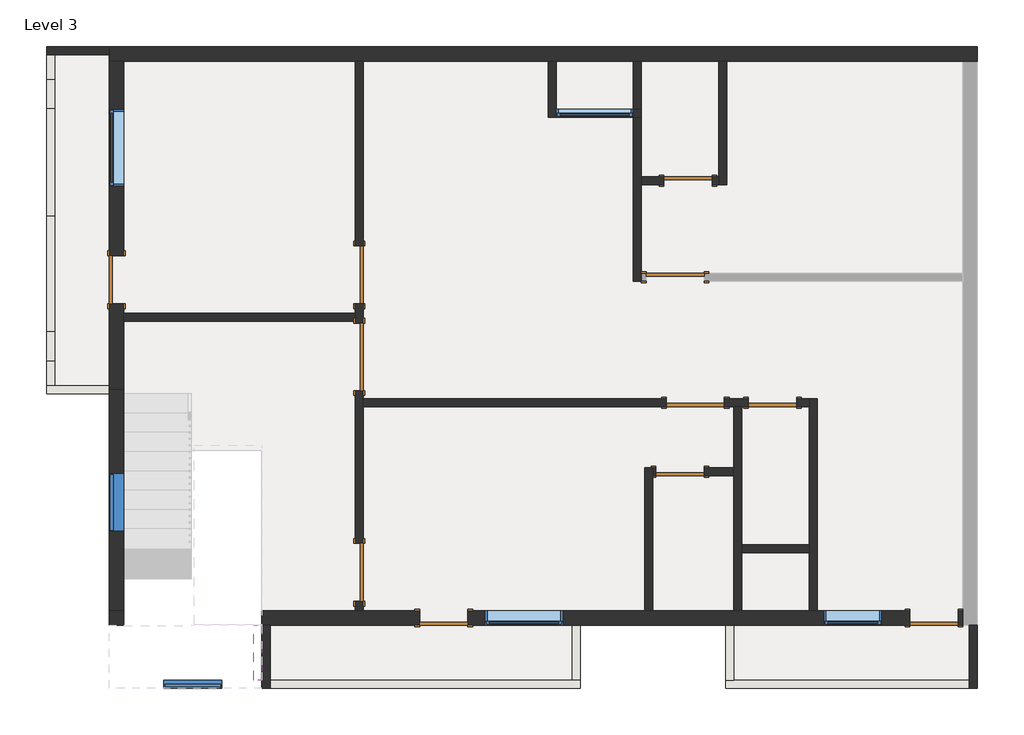
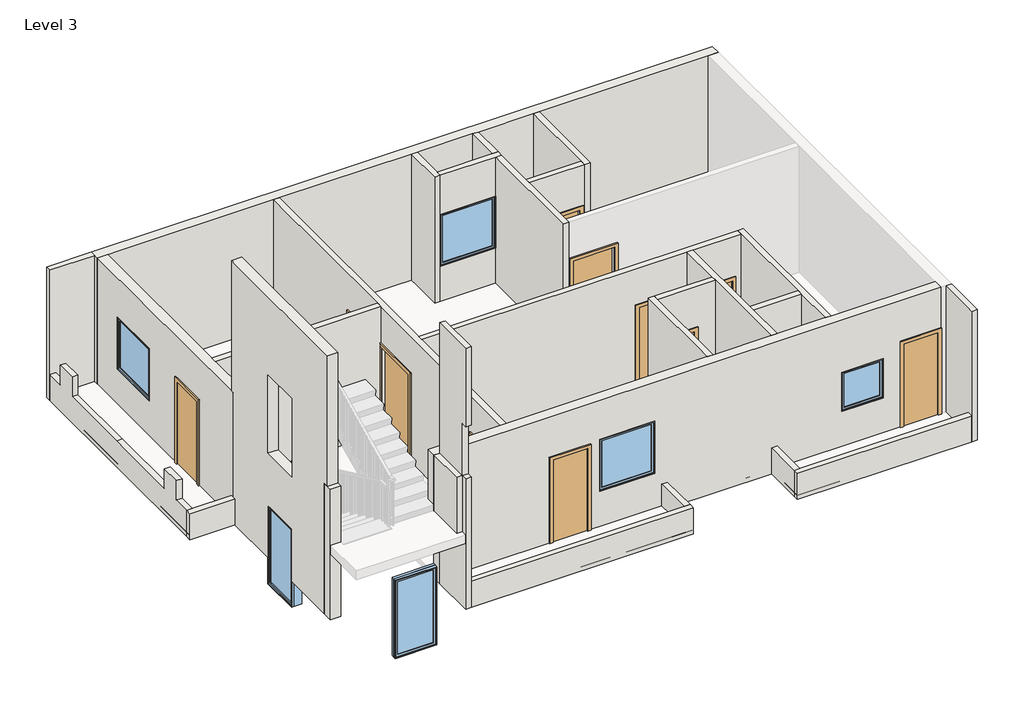
# One storey, part 1 of 2: 29 walls, 11 doors, 6 windows.
"""IFC4 building model written with IfcOpenShell, lengths in millimetres."""

from ifc_helpers import new_model, si_unit, frame, origin, place, context, project, spatial, polyline, outline, extrude, faceted_brep, transform, mapped, element, save
from components import door_1fe7f57d, door_85036156, door_a3eb833a, door_a1797ceb, door_4f94b823, window_6c5853a0, window_7da3115e, window_c796fc87, window_f887c457, window_76f305d9

model = new_model("IFC4")

# Units and contexts
model_context = context("Model", 3, world=origin())
ifc_project = project(units=[si_unit("LENGTHUNIT", "METRE", prefix="MILLI")], contexts=[model_context])

# Site, building, storey
site = spatial("IfcSite", under=ifc_project)
building = spatial("IfcBuilding", under=site)
storey = spatial("IfcBuildingStorey", under=building, Name="Level 3", Elevation=6096.0)

# Doors
placement = place(None, origin())
door_shape = door_1fe7f57d(model_context)
element("IfcDoor", 1, ObjectType="Single-Flush : 30\" x 80\"", at=placement, inside=storey, context=model_context, shape_type="MappedRepresentation", body=[
    mapped(door_shape, transform((-1197.7394758, 10653.5495492, 6096.0), x_axis=(1.0, 0.0, 0.0), y_axis=(0.0, 1.0, 0.0), z_axis=(0.0, 0.0, 1.0))),
])
element("IfcDoor", 2, ObjectType="Single-Flush : 30\" x 80\"", at=placement, inside=storey, context=model_context, shape_type="MappedRepresentation", body=[
    mapped(door_shape, transform((135.7605242, 7148.3495492, 6096.0), x_axis=(-1.0, 0.0, 0.0), y_axis=(0.0, -1.0, 0.0), z_axis=(0.0, 0.0, 1.0))),
])
element("IfcDoor", 3, ObjectType="Single-Flush : 30\" x 80\"", at=placement, inside=storey, context=model_context, shape_type="MappedRepresentation", body=[
    mapped(door_shape, transform((-1324.7394758, 6056.1495492, 6096.0), x_axis=(-1.0, 0.0, 0.0), y_axis=(0.0, -1.0, 0.0), z_axis=(0.0, 0.0, 1.0))),
])
door_2_shape = door_85036156(model_context)
element("IfcDoor", 4, ObjectType="Single-Flush : 30\" x 80\"", at=placement, inside=storey, context=model_context, shape_type="MappedRepresentation", body=[
    mapped(door_2_shape, transform((2688.4605242, 3744.7495492, 6096.0), x_axis=(1.0, 0.0, 0.0), y_axis=(0.0, 1.0, 0.0), z_axis=(0.0, 0.0, 1.0))),
])
element("IfcDoor", 5, ObjectType="Single-Flush : 30\" x 80\"", at=placement, inside=storey, context=model_context, shape_type="MappedRepresentation", body=[
    mapped(door_2_shape, transform((-5058.5394758, 3744.7495492, 6096.0), x_axis=(1.0, 0.0, 0.0), y_axis=(0.0, 1.0, 0.0), z_axis=(0.0, 0.0, 1.0))),
])
element("IfcDoor", 6, ObjectType="Single-Flush : 30\" x 80\"", at=placement, inside=storey, context=model_context, shape_type="MappedRepresentation", body=[
    mapped(door_2_shape, transform((-10227.4394758, 9091.4495492, 6096.0), x_axis=(0.0, -1.0, 0.0), y_axis=(1.0, 0.0, 0.0), z_axis=(0.0, 0.0, 1.0))),
])
door_3_shape = door_a3eb833a(model_context)
element("IfcDoor", 7, ObjectType="Single-Flush : 36\" x 84\"", at=placement, inside=storey, context=model_context, shape_type="MappedRepresentation", body=[
    mapped(door_3_shape, transform((-6392.0394758, 9167.6495492, 6096.0), x_axis=(0.0, 1.0, 0.0), y_axis=(-1.0, 0.0, 0.0), z_axis=(0.0, 0.0, 1.0))),
])
element("IfcDoor", 8, ObjectType="Single-Flush : 36\" x 84\"", at=placement, inside=storey, context=model_context, shape_type="MappedRepresentation", body=[
    mapped(door_3_shape, transform((-1400.9394758, 9129.5495492, 6096.0), x_axis=(-1.0, 0.0, 0.0), y_axis=(0.0, -1.0, 0.0), z_axis=(0.0, 0.0, 1.0))),
])
element("IfcDoor", 9, ObjectType="Single-Flush : 36\" x 84\"", at=placement, inside=storey, context=model_context, shape_type="MappedRepresentation", body=[
    mapped(door_3_shape, transform((-1083.4394758, 7148.3495492, 6096.0), x_axis=(1.0, 0.0, 0.0), y_axis=(0.0, 1.0, 0.0), z_axis=(0.0, 0.0, 1.0))),
])
door_4_shape = door_a1797ceb(model_context)
element("IfcDoor", 10, ObjectType="Single-Flush : 36\" x 84\"", at=placement, inside=storey, context=model_context, shape_type="MappedRepresentation", body=[
    mapped(door_4_shape, transform((-6392.0394758, 4468.6495492, 6096.0), x_axis=(0.0, -1.0, 0.0), y_axis=(1.0, 0.0, 0.0), z_axis=(0.0, 0.0, 1.0))),
])
door_5_shape = door_4f94b823(model_context)
element("IfcDoor", 11, ObjectType="Single-Flush : 42\" x 84\" 3,6\"", at=placement, inside=storey, context=model_context, shape_type="MappedRepresentation", body=[
    mapped(door_5_shape, transform((-6392.0394758, 7872.2495492, 6096.0), x_axis=(0.0, -1.0, 0.0), y_axis=(1.0, 0.0, 0.0), z_axis=(0.0, 0.0, 1.0))),
])

# Walls
element("IfcWall", 12, ObjectType="Generic - 5\"", at=placement, inside=storey, context=model_context, shape_type="Brep", body=[
    faceted_brep([(-6328.5394758, 4925.8495492, 6096.0), (-6328.5394758, 7084.8495492, 6096.0), (-6328.5394758, 7211.8495492, 6096.0), (-6328.5394758, 7338.8495492, 6096.0), (-6328.5394758, 7338.8495492, 8229.6), (-6328.5394758, 8405.6495492, 8229.6), (-6328.5394758, 8405.6495492, 6096.0), (-6328.5394758, 8710.4495492, 6096.0), (-6328.5394758, 8710.4495492, 8229.6), (-6328.5394758, 9624.8495492, 8229.6), (-6328.5394758, 9624.8495492, 6096.0), (-6328.5394758, 12545.8495492, 6096.0), (-6328.5394758, 12545.8495492, 9144.0), (-6328.5394758, 7211.8495492, 9144.0), (-6328.5394758, 7084.8495492, 9144.0), (-6328.5394758, 3859.0495492, 9144.0), (-6328.5394758, 3859.0495492, 6096.0), (-6328.5394758, 4011.4495492, 6096.0), (-6328.5394758, 4011.4495492, 8229.6), (-6328.5394758, 4925.8495492, 8229.6), (-6455.5394758, 7338.8495492, 8229.6), (-6455.5394758, 7338.8495492, 6096.0), (-6455.5394758, 4925.8495492, 6096.0), (-6455.5394758, 4925.8495492, 8229.6), (-6455.5394758, 4011.4495492, 8229.6), (-6455.5394758, 4011.4495492, 6096.0), (-6455.5394758, 3859.0495492, 6096.0), (-6455.5394758, 3859.0495492, 9144.0), (-6455.5394758, 8431.0495492, 9144.0), (-6455.5394758, 8558.0495492, 9144.0), (-6455.5394758, 12545.8495492, 9144.0), (-6455.5394758, 12545.8495492, 6096.0), (-6455.5394758, 9624.8495492, 6096.0), (-6455.5394758, 9624.8495492, 8229.6), (-6455.5394758, 8710.4495492, 8229.6), (-6455.5394758, 8710.4495492, 6096.0), (-6455.5394758, 8558.0495492, 6096.0), (-6455.5394758, 8431.0495492, 6096.0), (-6455.5394758, 8405.6495492, 6096.0), (-6455.5394758, 8405.6495492, 8229.6)], [[[0, 1, 2, 3, 4, 5, 6, 7, 8, 9, 10, 11, 12, 13, 14, 15, 16, 17, 18, 19]], [[20, 21, 22, 23, 24, 25, 26, 27, 28, 29, 30, 31, 32, 33, 34, 35, 36, 37, 38, 39]], [[11, 10, 32, 31]], [[26, 25, 17, 16]], [[22, 21, 3, 2, 1, 0]], [[38, 37, 36, 35, 7, 6]], [[15, 14, 13, 12, 30, 29, 28, 27]], [[16, 15, 27, 26]], [[12, 11, 31, 30]], [[33, 32, 10, 9]], [[34, 33, 9, 8]], [[35, 34, 8, 7]], [[18, 17, 25, 24]], [[19, 18, 24, 23]], [[0, 19, 23, 22]], [[4, 3, 21, 20]], [[5, 4, 20, 39]], [[6, 5, 39, 38]]]),
])
element("IfcWall", 13, ObjectType="Generic - 5\"", at=placement, inside=storey, context=model_context, shape_type="SweptSolid", body=[
    extrude(outline(polyline([(-10113.1394758, 8558.0495492), (-6455.5394758, 8558.0495492), (-6455.5394758, 8431.0495492), (-10113.1394758, 8431.0495492), (-10113.1394758, 8558.0495492)])), frame((0.0, 0.0, 6096.0), z_axis=(0.0, 0.0, 1.0), x_axis=(1.0, 0.0, 0.0)), (0.0, 0.0, 1.0), 3048.0),
])
element("IfcWall", 14, ObjectType="Generic - 5\"", at=placement, inside=storey, context=model_context, shape_type="Brep", body=[
    faceted_brep([(-245.2394758, 7211.8495492, 8128.0), (-245.2394758, 7211.8495492, 6096.0), (-626.2394758, 7211.8495492, 6096.0), (-626.2394758, 7211.8495492, 8229.6), (-1540.6394758, 7211.8495492, 8229.6), (-1540.6394758, 7211.8495492, 6096.0), (-6328.5394758, 7211.8495492, 6096.0), (-6328.5394758, 7211.8495492, 9144.0), (719.9605242, 7211.8495492, 9144.0), (719.9605242, 7211.8495492, 6096.0), (516.7605242, 7211.8495492, 6096.0), (516.7605242, 7211.8495492, 8128.0), (-626.2394758, 7084.8495492, 6096.0), (-473.8394758, 7084.8495492, 6096.0), (-346.8394758, 7084.8495492, 6096.0), (-245.2394758, 7084.8495492, 6096.0), (-245.2394758, 7084.8495492, 8128.0), (516.7605242, 7084.8495492, 8128.0), (516.7605242, 7084.8495492, 6096.0), (719.9605242, 7084.8495492, 6096.0), (719.9605242, 7084.8495492, 9144.0), (-346.8394758, 7084.8495492, 9144.0), (-473.8394758, 7084.8495492, 9144.0), (-6328.5394758, 7084.8495492, 9144.0), (-6328.5394758, 7084.8495492, 6096.0), (-1540.6394758, 7084.8495492, 6096.0), (-1540.6394758, 7084.8495492, 8229.6), (-626.2394758, 7084.8495492, 8229.6)], [[[0, 1, 2, 3, 4, 5, 6, 7, 8, 9, 10, 11]], [[12, 13, 14, 15, 16, 17, 18, 19, 20, 21, 22, 23, 24, 25, 26, 27]], [[25, 24, 6, 5]], [[10, 9, 19, 18]], [[2, 1, 15, 14, 13, 12]], [[8, 7, 23, 22, 21, 20]], [[7, 6, 24, 23]], [[9, 8, 20, 19]], [[3, 2, 12, 27]], [[4, 3, 27, 26]], [[5, 4, 26, 25]], [[16, 15, 1, 0]], [[17, 16, 0, 11]], [[18, 17, 11, 10]]]),
])
element("IfcWall", 15, ObjectType="Generic - 5\"", at=placement, inside=storey, context=model_context, shape_type="Brep", body=[
    faceted_brep([(-2061.3394758, 11656.8495492, 6096.0), (-2061.3394758, 9066.0495492, 6096.0), (-2061.3394758, 9066.0495492, 9144.0), (-2061.3394758, 11656.8495492, 9144.0), (-1934.3394758, 11656.8495492, 6096.0), (-1934.3394758, 11656.8495492, 9144.0), (-1934.3394758, 10717.0495492, 9144.0), (-1934.3394758, 10590.0495492, 9144.0), (-1934.3394758, 9193.0495492, 9144.0), (-1934.3394758, 9066.0495492, 9144.0), (-1934.3394758, 9066.0495492, 6096.0), (-1934.3394758, 9193.0495492, 6096.0), (-1934.3394758, 10590.0495492, 6096.0), (-1934.3394758, 10717.0495492, 6096.0)], [[[0, 1, 2, 3]], [[4, 5, 6, 7, 8, 9, 10, 11, 12, 13]], [[1, 0, 4, 13, 12, 11, 10]], [[3, 2, 9, 8, 7, 6, 5]], [[0, 3, 5, 4]], [[2, 1, 10, 9]]]),
])
element("IfcWall", 16, ObjectType="Generic - 5\"", at=placement, inside=storey, context=model_context, shape_type="Brep", body=[
    faceted_brep([(-346.8394758, 3859.0495492, 6096.0), (-346.8394758, 4773.4495492, 6096.0), (-346.8394758, 4900.4495492, 6096.0), (-346.8394758, 7084.8495492, 6096.0), (-346.8394758, 7084.8495492, 9144.0), (-346.8394758, 4900.4495492, 9144.0), (-346.8394758, 4773.4495492, 9144.0), (-346.8394758, 3859.0495492, 9144.0), (-473.8394758, 3859.0495492, 6096.0), (-473.8394758, 3859.0495492, 9144.0), (-473.8394758, 5992.6495492, 9144.0), (-473.8394758, 6119.6495492, 9144.0), (-473.8394758, 7084.8495492, 9144.0), (-473.8394758, 7084.8495492, 6096.0), (-473.8394758, 6119.6495492, 6096.0), (-473.8394758, 5992.6495492, 6096.0)], [[[0, 1, 2, 3, 4, 5, 6, 7]], [[8, 9, 10, 11, 12, 13, 14, 15]], [[3, 2, 1, 0, 8, 15, 14, 13]], [[7, 6, 5, 4, 12, 11, 10, 9]], [[4, 3, 13, 12]], [[0, 7, 9, 8]]]),
])
element("IfcWall", 17, ObjectType="Generic - 5\"", at=placement, inside=storey, context=model_context, shape_type="Brep", body=[
    faceted_brep([(846.9605242, 3859.0495492, 6096.0), (846.9605242, 7211.8495492, 6096.0), (846.9605242, 7211.8495492, 9144.0), (846.9605242, 3859.0495492, 9144.0), (719.9605242, 3859.0495492, 6096.0), (719.9605242, 3859.0495492, 9144.0), (719.9605242, 4773.4495492, 9144.0), (719.9605242, 4900.4495492, 9144.0), (719.9605242, 7084.8495492, 9144.0), (719.9605242, 7211.8495492, 9144.0), (719.9605242, 7211.8495492, 6096.0), (719.9605242, 7084.8495492, 6096.0), (719.9605242, 4900.4495492, 6096.0), (719.9605242, 4773.4495492, 6096.0)], [[[0, 1, 2, 3]], [[4, 5, 6, 7, 8, 9, 10, 11, 12, 13]], [[1, 0, 4, 13, 12, 11, 10]], [[3, 2, 9, 8, 7, 6, 5]], [[0, 3, 5, 4]], [[2, 1, 10, 9]]]),
])
element("IfcWall", 18, ObjectType="Generic - 5\"", at=placement, inside=storey, context=model_context, shape_type="Brep", body=[
    faceted_brep([(-1756.5394758, 3859.0495492, 6096.0), (-1756.5394758, 5992.6495492, 6096.0), (-1756.5394758, 6119.6495492, 6096.0), (-1756.5394758, 6119.6495492, 9144.0), (-1756.5394758, 5992.6495492, 9144.0), (-1756.5394758, 3859.0495492, 9144.0), (-1883.5394758, 3859.0495492, 6096.0), (-1883.5394758, 3859.0495492, 9144.0), (-1883.5394758, 6119.6495492, 9144.0), (-1883.5394758, 6119.6495492, 6096.0)], [[[0, 1, 2, 3, 4, 5]], [[6, 7, 8, 9]], [[2, 1, 0, 6, 9]], [[5, 4, 3, 8, 7]], [[0, 5, 7, 6]], [[3, 2, 9, 8]]]),
])
element("IfcWall", 19, ObjectType="Generic - 5\"", at=placement, inside=storey, context=model_context, shape_type="SweptSolid", body=[
    extrude(outline(polyline([(6096.0, -1756.5394758), (6096.0, -1705.7394758), (8128.0, -1705.7394758), (8128.0, -943.7394758), (6096.0, -943.7394758), (6096.0, -473.8394758), (9144.0, -473.8394758), (9144.0, -1756.5394758), (6096.0, -1756.5394758)])), frame((0.0, 5992.6495492, 0.0), z_axis=(0.0, 1.0, 0.0), x_axis=(0.0, 0.0, 1.0)), (0.0, 0.0, 1.0), 127.0),
])
element("IfcWall", 20, ObjectType="Generic - 5\"", at=placement, inside=storey, context=model_context, shape_type="SweptSolid", body=[
    extrude(outline(polyline([(719.9605242, 4773.4495492), (-346.8394758, 4773.4495492), (-346.8394758, 4900.4495492), (719.9605242, 4900.4495492), (719.9605242, 4773.4495492)])), frame((0.0, 0.0, 6096.0), z_axis=(0.0, 0.0, 1.0), x_axis=(1.0, 0.0, 0.0)), (0.0, 0.0, 1.0), 3048.0),
])
element("IfcWall", 21, ObjectType="Generic - 5\"", at=placement, inside=storey, context=model_context, shape_type="Brep", body=[
    faceted_brep([(-715.1394758, 12545.8495492, 6096.0), (-715.1394758, 10717.0495492, 6096.0), (-715.1394758, 10590.0495492, 6096.0), (-715.1394758, 10590.0495492, 9144.0), (-715.1394758, 10717.0495492, 9144.0), (-715.1394758, 12545.8495492, 9144.0), (-588.1394758, 12545.8495492, 6096.0), (-588.1394758, 12545.8495492, 9144.0), (-588.1394758, 10590.0495492, 9144.0), (-588.1394758, 10590.0495492, 6096.0)], [[[0, 1, 2, 3, 4, 5]], [[6, 7, 8, 9]], [[2, 1, 0, 6, 9]], [[5, 4, 3, 8, 7]], [[0, 5, 7, 6]], [[3, 2, 9, 8]]]),
])
element("IfcWall", 22, ObjectType="Generic - 5\"", at=placement, inside=storey, context=model_context, shape_type="SweptSolid", body=[
    extrude(outline(polyline([(8128.0, -816.7394758), (6096.0, -816.7394758), (6096.0, -715.1394758), (9144.0, -715.1394758), (9144.0, -1934.3394758), (6096.0, -1934.3394758), (6096.0, -1578.7394758), (8128.0, -1578.7394758), (8128.0, -816.7394758)])), frame((0.0, 10590.0495492, 0.0), z_axis=(0.0, 1.0, 0.0), x_axis=(0.0, 0.0, 1.0)), (0.0, 0.0, 1.0), 127.0),
])
element("IfcWall", 23, ObjectType="Generic - 5\"", at=placement, inside=storey, context=model_context, shape_type="Brep", body=[
    faceted_brep([(-3407.5394758, 12545.8495492, 6096.0), (-3407.5394758, 11656.8495492, 6096.0), (-3407.5394758, 11656.8495492, 9144.0), (-3407.5394758, 12545.8495492, 9144.0), (-3280.5394758, 12545.8495492, 6096.0), (-3280.5394758, 12545.8495492, 9144.0), (-3280.5394758, 11783.8495492, 9144.0), (-3280.5394758, 11656.8495492, 9144.0), (-3280.5394758, 11656.8495492, 6096.0), (-3280.5394758, 11783.8495492, 6096.0)], [[[0, 1, 2, 3]], [[4, 5, 6, 7, 8, 9]], [[1, 0, 4, 9, 8]], [[3, 2, 7, 6, 5]], [[0, 3, 5, 4]], [[2, 1, 8, 7]]]),
])
element("IfcWall", 24, ObjectType="Generic - 5\"", at=placement, inside=storey, context=model_context, shape_type="Brep", body=[
    faceted_brep([(-2061.3394758, 11656.8495492, 7010.4), (-3280.5394758, 11656.8495492, 7010.4), (-3280.5394758, 11656.8495492, 6096.0), (-2061.3394758, 11656.8495492, 6096.0), (-1934.3394758, 11656.8495492, 6096.0), (-1934.3394758, 11656.8495492, 9144.0), (-2061.3394758, 11656.8495492, 9144.0), (-3280.5394758, 11656.8495492, 9144.0), (-3280.5394758, 11656.8495492, 8229.6), (-2061.3394758, 11656.8495492, 8229.6), (-3280.5394758, 11783.8495492, 6096.0), (-3280.5394758, 11783.8495492, 7010.4), (-2061.3394758, 11783.8495492, 7010.4), (-2061.3394758, 11783.8495492, 8229.6), (-3280.5394758, 11783.8495492, 8229.6), (-3280.5394758, 11783.8495492, 9144.0), (-2061.3394758, 11783.8495492, 9144.0), (-1934.3394758, 11783.8495492, 9144.0), (-1934.3394758, 11783.8495492, 6096.0), (-2061.3394758, 11783.8495492, 6096.0)], [[[0, 1, 2, 3, 4, 5, 6, 7, 8, 9]], [[10, 11, 12, 13, 14, 15, 16, 17, 18, 19]], [[4, 3, 2, 10, 19, 18]], [[7, 6, 5, 17, 16, 15]], [[8, 7, 15, 14]], [[2, 1, 11, 10]], [[5, 4, 18, 17]], [[12, 11, 1, 0]], [[13, 12, 0, 9]], [[14, 13, 9, 8]]]),
])
element("IfcWall", 25, ObjectType="Generic - 5\"", at=placement, inside=storey, context=model_context, shape_type="SweptSolid", body=[
    extrude(outline(polyline([(-1934.3394758, 12545.8495492), (-1934.3394758, 11783.8495492), (-2061.3394758, 11783.8495492), (-2061.3394758, 12545.8495492), (-1934.3394758, 12545.8495492)])), frame((0.0, 0.0, 6096.0), z_axis=(0.0, 0.0, 1.0), x_axis=(1.0, 0.0, 0.0)), (0.0, 0.0, 1.0), 3048.0),
])
element("IfcWall", 26, ObjectType="Generic - 5\"", at=placement, inside=storey, context=model_context, shape_type="SweptSolid", body=[
    extrude(outline(polyline([(-7928.7394758, 3630.4495492), (-7928.7394758, 2766.8495492), (-8055.7394758, 2766.8495492), (-8055.7394758, 3630.4495492), (-7928.7394758, 3630.4495492)])), frame((0.0, 0.0, 7634.5142857), z_axis=(0.0, 0.0, 1.0), x_axis=(1.0, 0.0, 0.0)), (0.0, 0.0, 1.0), 1509.4857143),
])
element("IfcWall", 27, ObjectType="Generic - 5\"", at=placement, inside=storey, context=model_context, shape_type="Brep", body=[
    faceted_brep([(3247.2605242, 3630.4495492, 6096.0), (3247.2605242, 2766.8495492, 6096.0), (3247.2605242, 2639.8495492, 6096.0), (3247.2605242, 2639.8495492, 6705.6), (3247.2605242, 2639.8495492, 9144.0), (3247.2605242, 3630.4495492, 9144.0), (3374.2605242, 3630.4495492, 6096.0), (3374.2605242, 3630.4495492, 9144.0), (3374.2605242, 2639.8495492, 9144.0), (3374.2605242, 2639.8495492, 6096.0)], [[[0, 1, 2, 3, 4, 5]], [[6, 7, 8, 9]], [[2, 1, 0, 6, 9]], [[5, 4, 8, 7]], [[4, 3, 2, 9, 8]], [[0, 5, 7, 6]]]),
])
element("IfcWall", 28, ObjectType="Generic - 5\"", at=placement, inside=storey, context=model_context, shape_type="Brep", body=[
    faceted_brep([(3247.2605242, 2766.8495492, 6096.0), (-473.8394758, 2766.8495492, 6096.0), (-600.8394758, 2766.8495492, 6096.0), (-600.8394758, 2766.8495492, 6705.6), (-473.8394758, 2766.8495492, 6705.6), (3247.2605242, 2766.8495492, 6705.6), (3247.2605242, 2639.8495492, 6096.0), (3247.2605242, 2639.8495492, 6705.6), (-600.8394758, 2639.8495492, 6705.6), (-600.8394758, 2639.8495492, 6096.0)], [[[0, 1, 2, 3, 4, 5]], [[6, 7, 8, 9]], [[2, 1, 0, 6, 9]], [[5, 4, 3, 8, 7]], [[0, 5, 7, 6]], [[3, 2, 9, 8]]]),
])
element("IfcWall", 29, ObjectType="Generic - 5\"", at=placement, inside=storey, context=model_context, shape_type="SweptSolid", body=[
    extrude(outline(polyline([(-473.8394758, 3630.4495492), (-473.8394758, 2766.8495492), (-600.8394758, 2766.8495492), (-600.8394758, 3630.4495492), (-473.8394758, 3630.4495492)])), frame((0.0, 0.0, 6096.0), z_axis=(0.0, 0.0, 1.0), x_axis=(1.0, 0.0, 0.0)), (0.0, 0.0, 1.0), 609.6),
])
element("IfcWall", 30, ObjectType="Generic - 5\"", at=placement, inside=storey, context=model_context, shape_type="Brep", body=[
    faceted_brep([(-7928.7394758, 3630.4495492, 6096.0), (-7928.7394758, 2639.8495492, 6096.0), (-7928.7394758, 2639.8495492, 9144.0), (-7928.7394758, 2766.8495492, 9144.0), (-7928.7394758, 2766.8495492, 10363.2), (-7928.7394758, 2639.8495492, 10363.2), (-7928.7394758, 2639.8495492, 12192.0), (-7928.7394758, 2766.8495492, 12192.0), (-7928.7394758, 3630.4495492, 12192.0), (-7928.7394758, 3630.4495492, 9144.0), (-7928.7394758, 3630.4495492, 7634.5142857), (-7801.7394758, 3630.4495492, 6096.0), (-7801.7394758, 3630.4495492, 12192.0), (-7801.7394758, 2639.8495492, 12192.0), (-7801.7394758, 2639.8495492, 10363.2), (-7801.7394758, 2766.8495492, 10363.2), (-7801.7394758, 2766.8495492, 9144.0), (-7801.7394758, 2639.8495492, 9144.0), (-7801.7394758, 2639.8495492, 6705.6), (-7801.7394758, 2639.8495492, 6096.0), (-7801.7394758, 2766.8495492, 6096.0)], [[[0, 1, 2, 3, 4, 5, 6, 7, 8, 9, 10]], [[11, 12, 13, 14, 15, 16, 17, 18, 19, 20]], [[1, 0, 11, 20, 19]], [[8, 7, 6, 13, 12]], [[0, 10, 9, 8, 12, 11]], [[16, 3, 2, 17]], [[14, 5, 4, 15]], [[1, 19, 18, 17, 2]], [[4, 3, 16, 15]], [[6, 5, 14, 13]]]),
])
element("IfcWall", 31, ObjectType="Generic - 5\"", at=placement, inside=storey, context=model_context, shape_type="Brep", body=[
    faceted_brep([(-7801.7394758, 2639.8495492, 6096.0), (-2899.5394758, 2639.8495492, 6096.0), (-2899.5394758, 2639.8495492, 6705.6), (-7801.7394758, 2639.8495492, 6705.6), (-7801.7394758, 2766.8495492, 6096.0), (-7801.7394758, 2766.8495492, 6705.6), (-3026.5394758, 2766.8495492, 6705.6), (-2899.5394758, 2766.8495492, 6705.6), (-2899.5394758, 2766.8495492, 6096.0), (-3026.5394758, 2766.8495492, 6096.0)], [[[0, 1, 2, 3]], [[4, 5, 6, 7, 8, 9]], [[1, 0, 4, 9, 8]], [[3, 2, 7, 6, 5]], [[2, 1, 8, 7]], [[0, 3, 5, 4]]]),
])
element("IfcWall", 32, ObjectType="Generic - 5\"", at=placement, inside=storey, context=model_context, shape_type="SweptSolid", body=[
    extrude(outline(polyline([(-2899.5394758, 3630.4495492), (-2899.5394758, 2766.8495492), (-3026.5394758, 2766.8495492), (-3026.5394758, 3630.4495492), (-2899.5394758, 3630.4495492)])), frame((0.0, 0.0, 6096.0), z_axis=(0.0, 0.0, 1.0), x_axis=(1.0, 0.0, 0.0)), (0.0, 0.0, 1.0), 609.6),
])
element("IfcWall", 33, ObjectType="Generic - 5\"", at=placement, inside=storey, context=model_context, shape_type="Brep", body=[
    faceted_brep([(-10341.7394758, 12774.4495492, 6096.0), (-11332.3394758, 12774.4495492, 6096.0), (-11332.3394758, 12774.4495492, 9144.0), (-10341.7394758, 12774.4495492, 9144.0), (-10341.7394758, 12647.4495492, 6096.0), (-10341.7394758, 12647.4495492, 9144.0), (-11332.3394758, 12647.4495492, 9144.0), (-11332.3394758, 12647.4495492, 6705.6), (-11332.3394758, 12647.4495492, 6096.0), (-11205.3394758, 12647.4495492, 6096.0)], [[[0, 1, 2, 3]], [[4, 5, 6, 7, 8, 9]], [[1, 0, 4, 9, 8]], [[3, 2, 6, 5]], [[0, 3, 5, 4]], [[2, 1, 8, 7, 6]]]),
])
element("IfcWall", 34, ObjectType="Generic - 5\"", at=placement, inside=storey, context=model_context, shape_type="Brep", body=[
    faceted_brep([(-11332.3394758, 7288.0495492, 6096.0), (-10341.7394758, 7288.0495492, 6096.0), (-10341.7394758, 7288.0495492, 6705.6), (-11332.3394758, 7288.0495492, 6705.6), (-11332.3394758, 7415.0495492, 6096.0), (-11332.3394758, 7415.0495492, 6705.6), (-11205.3394758, 7415.0495492, 6705.6), (-10341.7394758, 7415.0495492, 6705.6), (-10341.7394758, 7415.0495492, 6096.0), (-11205.3394758, 7415.0495492, 6096.0), (-10341.7394758, 7351.5495492, 6096.0)], [[[0, 1, 2, 3]], [[4, 5, 6, 7, 8, 9]], [[1, 0, 4, 9, 8, 10]], [[3, 2, 7, 6, 5]], [[2, 1, 10, 8, 7]], [[0, 3, 5, 4]]]),
])
element("IfcWall", 35, ObjectType="Generic - 5\"", at=placement, inside=storey, context=model_context, shape_type="SweptSolid", body=[
    extrude(outline(polyline([(12647.4495492, 6096.0), (7415.0495492, 6096.0), (7415.0495492, 6705.6), (7808.7495492, 6705.6), (7808.7495492, 7162.8), (8265.9495492, 7162.8), (8265.9495492, 6705.6), (10094.7495492, 6705.6), (11796.5495492, 6705.6), (11796.5495492, 7162.8), (12253.7495492, 7162.8), (12253.7495492, 6705.6), (12647.4495492, 6705.6), (12647.4495492, 6096.0)])), frame((-11332.3394758, 0.0, 0.0), z_axis=(1.0, 0.0, 0.0), x_axis=(0.0, 1.0, 0.0)), (0.0, 0.0, 1.0), 127.0),
])
element("IfcWall", 36, ObjectType="Generic - 9\"", at=placement, inside=storey, context=model_context, shape_type="Brep", body=[
    faceted_brep([(-10341.7394758, 12545.8495492, 6096.0), (-10113.1394758, 12545.8495492, 6096.0), (-6455.5394758, 12545.8495492, 6096.0), (-6328.5394758, 12545.8495492, 6096.0), (-3407.5394758, 12545.8495492, 6096.0), (-3280.5394758, 12545.8495492, 6096.0), (-2061.3394758, 12545.8495492, 6096.0), (-1934.3394758, 12545.8495492, 6096.0), (-715.1394758, 12545.8495492, 6096.0), (-588.1394758, 12545.8495492, 6096.0), (3145.6605242, 12545.8495492, 6096.0), (3374.2605242, 12545.8495492, 6096.0), (3374.2605242, 12545.8495492, 9144.0), (3145.6605242, 12545.8495492, 9144.0), (-588.1394758, 12545.8495492, 9144.0), (-715.1394758, 12545.8495492, 9144.0), (-1934.3394758, 12545.8495492, 9144.0), (-2061.3394758, 12545.8495492, 9144.0), (-3280.5394758, 12545.8495492, 9144.0), (-3407.5394758, 12545.8495492, 9144.0), (-6328.5394758, 12545.8495492, 9144.0), (-6455.5394758, 12545.8495492, 9144.0), (-10113.1394758, 12545.8495492, 9144.0), (-10341.7394758, 12545.8495492, 9144.0), (-10341.7394758, 12774.4495492, 6096.0), (-10341.7394758, 12774.4495492, 9144.0), (3374.2605242, 12774.4495492, 9144.0), (3374.2605242, 12774.4495492, 6096.0), (-10341.7394758, 12647.4495492, 6096.0), (-10341.7394758, 12647.4495492, 9144.0)], [[[0, 1, 2, 3, 4, 5, 6, 7, 8, 9, 10, 11, 12, 13, 14, 15, 16, 17, 18, 19, 20, 21, 22, 23]], [[24, 25, 26, 27]], [[11, 10, 9, 8, 7, 6, 5, 4, 3, 2, 1, 0, 28, 24, 27]], [[23, 22, 21, 20, 19, 18, 17, 16, 15, 14, 13, 12, 26, 25, 29]], [[12, 11, 27, 26]], [[0, 23, 29, 25, 24, 28]]]),
])
element("IfcWall", 37, ObjectType="Generic - 9\"", at=placement, inside=storey, context=model_context, shape_type="Brep", body=[
    faceted_brep([(2307.4605242, 3859.0495492, 6096.0), (846.9605242, 3859.0495492, 6096.0), (719.9605242, 3859.0495492, 6096.0), (-346.8394758, 3859.0495492, 6096.0), (-473.8394758, 3859.0495492, 6096.0), (-1756.5394758, 3859.0495492, 6096.0), (-1883.5394758, 3859.0495492, 6096.0), (-4677.5394758, 3859.0495492, 6096.0), (-4677.5394758, 3859.0495492, 8128.0), (-5439.5394758, 3859.0495492, 8128.0), (-5439.5394758, 3859.0495492, 6096.0), (-6328.5394758, 3859.0495492, 6096.0), (-6455.5394758, 3859.0495492, 6096.0), (-7928.7394758, 3859.0495492, 6096.0), (-7928.7394758, 3859.0495492, 7634.5142857), (-8055.7394758, 3859.0495492, 7634.5142857), (-8055.7394758, 3859.0495492, 9144.0), (-6455.5394758, 3859.0495492, 9144.0), (-6328.5394758, 3859.0495492, 9144.0), (-1883.5394758, 3859.0495492, 9144.0), (-1756.5394758, 3859.0495492, 9144.0), (-473.8394758, 3859.0495492, 9144.0), (-346.8394758, 3859.0495492, 9144.0), (719.9605242, 3859.0495492, 9144.0), (846.9605242, 3859.0495492, 9144.0), (3145.6605242, 3859.0495492, 9144.0), (3145.6605242, 3859.0495492, 6096.0), (3069.4605242, 3859.0495492, 6096.0), (3069.4605242, 3859.0495492, 8128.0), (2307.4605242, 3859.0495492, 8128.0), (-4398.1394758, 3859.0495492, 8229.6), (-4398.1394758, 3859.0495492, 7010.4), (-3178.9394758, 3859.0495492, 7010.4), (-3178.9394758, 3859.0495492, 8229.6), (948.5605242, 3859.0495492, 7924.8), (948.5605242, 3859.0495492, 7010.4), (1862.9605242, 3859.0495492, 7010.4), (1862.9605242, 3859.0495492, 7924.8), (-4677.5394758, 3630.4495492, 8128.0), (-4677.5394758, 3630.4495492, 6096.0), (-3026.5394758, 3630.4495492, 6096.0), (-2899.5394758, 3630.4495492, 6096.0), (-600.8394758, 3630.4495492, 6096.0), (-473.8394758, 3630.4495492, 6096.0), (2307.4605242, 3630.4495492, 6096.0), (2307.4605242, 3630.4495492, 8128.0), (3069.4605242, 3630.4495492, 8128.0), (3069.4605242, 3630.4495492, 6096.0), (3145.6605242, 3630.4495492, 6096.0), (3145.6605242, 3630.4495492, 9144.0), (-7928.7394758, 3630.4495492, 9144.0), (-8055.7394758, 3630.4495492, 9144.0), (-8055.7394758, 3630.4495492, 7634.5142857), (-7928.7394758, 3630.4495492, 7634.5142857), (-7928.7394758, 3630.4495492, 6096.0), (-7801.7394758, 3630.4495492, 6096.0), (-5439.5394758, 3630.4495492, 6096.0), (-5439.5394758, 3630.4495492, 8128.0), (-4398.1394758, 3630.4495492, 8229.6), (-3178.9394758, 3630.4495492, 8229.6), (-3178.9394758, 3630.4495492, 7010.4), (-4398.1394758, 3630.4495492, 7010.4), (948.5605242, 3630.4495492, 7924.8), (1862.9605242, 3630.4495492, 7924.8), (1862.9605242, 3630.4495492, 7010.4), (948.5605242, 3630.4495492, 7010.4)], [[[0, 1, 2, 3, 4, 5, 6, 7, 8, 9, 10, 11, 12, 13, 14, 15, 16, 17, 18, 19, 20, 21, 22, 23, 24, 25, 26, 27, 28, 29], [30, 31, 32, 33], [34, 35, 36, 37]], [[38, 39, 40, 41, 42, 43, 44, 45, 46, 47, 48, 49, 50, 51, 52, 53, 54, 55, 56, 57], [58, 59, 60, 61], [62, 63, 64, 65]], [[48, 47, 27, 26]], [[56, 55, 54, 13, 12, 11, 10]], [[44, 43, 42, 41, 40, 39, 7, 6, 5, 4, 3, 2, 1, 0]], [[25, 24, 23, 22, 21, 20, 19, 18, 17, 16, 51, 50, 49]], [[26, 25, 49, 48]], [[52, 15, 14, 53]], [[16, 15, 52, 51]], [[14, 13, 54, 53]], [[31, 30, 58, 61]], [[32, 31, 61, 60]], [[33, 32, 60, 59]], [[30, 33, 59, 58]], [[35, 34, 62, 65]], [[36, 35, 65, 64]], [[37, 36, 64, 63]], [[34, 37, 63, 62]], [[28, 27, 47, 46]], [[29, 28, 46, 45]], [[0, 29, 45, 44]], [[8, 7, 39, 38]], [[9, 8, 38, 57]], [[10, 9, 57, 56]]]),
])
element("IfcWall", 38, ObjectType="Generic - 9\"", at=placement, inside=storey, context=model_context, shape_type="Brep", body=[
    faceted_brep([(-10113.1394758, 7415.0495492, 12192.0), (-10113.1394758, 3744.7495492, 12192.0), (-10113.1394758, 3744.7495492, 9144.0), (-10113.1394758, 3859.0495492, 9144.0), (-10113.1394758, 3859.0495492, 6096.0), (-10113.1394758, 5116.3495492, 6096.0), (-10113.1394758, 5116.3495492, 7315.2), (-10113.1394758, 6030.7495492, 7315.2), (-10113.1394758, 6030.7495492, 6096.0), (-10113.1394758, 7351.5495492, 6096.0), (-10113.1394758, 7351.5495492, 9144.0), (-10113.1394758, 7415.0495492, 9144.0), (-10113.1394758, 6030.7495492, 10363.2), (-10113.1394758, 6030.7495492, 8534.4), (-10113.1394758, 5116.3495492, 8534.4), (-10113.1394758, 5116.3495492, 10363.2), (-10341.7394758, 3744.7495492, 12192.0), (-10341.7394758, 7288.0495492, 12192.0), (-10341.7394758, 7415.0495492, 12192.0), (-10341.7394758, 7415.0495492, 9144.0), (-10341.7394758, 7351.5495492, 9144.0), (-10341.7394758, 7351.5495492, 6096.0), (-10341.7394758, 7288.0495492, 6096.0), (-10341.7394758, 6030.7495492, 6096.0), (-10341.7394758, 6030.7495492, 7315.2), (-10341.7394758, 5116.3495492, 7315.2), (-10341.7394758, 5116.3495492, 6096.0), (-10341.7394758, 3859.0495492, 6096.0), (-10341.7394758, 3859.0495492, 9144.0), (-10341.7394758, 3744.7495492, 9144.0), (-10341.7394758, 6030.7495492, 10363.2), (-10341.7394758, 5116.3495492, 10363.2), (-10341.7394758, 5116.3495492, 8534.4), (-10341.7394758, 6030.7495492, 8534.4), (-10214.7394758, 3744.7495492, 12192.0), (-10214.7394758, 3744.7495492, 9144.0)], [[[0, 1, 2, 3, 4, 5, 6, 7, 8, 9, 10, 11], [12, 13, 14, 15]], [[16, 17, 18, 19, 20, 21, 22, 23, 24, 25, 26, 27, 28, 29], [30, 31, 32, 33]], [[4, 27, 26, 5]], [[21, 9, 8, 23, 22]], [[1, 0, 18, 17, 16, 34]], [[1, 34, 16, 29, 35, 2]], [[27, 4, 3, 28]], [[9, 21, 20, 10]], [[11, 10, 20, 19]], [[0, 11, 19, 18]], [[2, 35, 29, 28, 3]], [[7, 24, 23, 8]], [[25, 6, 5, 26]], [[24, 7, 6, 25]], [[13, 12, 30, 33]], [[14, 13, 33, 32]], [[15, 14, 32, 31]], [[12, 15, 31, 30]]]),
])
element("IfcWall", 39, ObjectType="Generic - 9\"", at=placement, inside=storey, context=model_context, shape_type="Brep", body=[
    faceted_brep([(-10113.1394758, 3859.0495492, 6096.0), (-10341.7394758, 3859.0495492, 6096.0), (-10341.7394758, 3859.0495492, 9144.0), (-10113.1394758, 3859.0495492, 9144.0), (-10113.1394758, 3630.4495492, 6096.0), (-10113.1394758, 3630.4495492, 9144.0), (-10214.7394758, 3630.4495492, 9144.0), (-10341.7394758, 3630.4495492, 9144.0), (-10341.7394758, 3630.4495492, 6096.0), (-10341.7394758, 3744.7495492, 9144.0)], [[[0, 1, 2, 3]], [[4, 5, 6, 7, 8]], [[1, 0, 4, 8]], [[3, 2, 9, 7, 6, 5]], [[0, 3, 5, 4]], [[2, 1, 8, 7, 9]]]),
])
element("IfcWall", 40, ObjectType="Generic - 9\"", at=placement, inside=storey, context=model_context, shape_type="Brep", body=[
    faceted_brep([(-10113.1394758, 7351.5495492, 6096.0), (-10113.1394758, 8431.0495492, 6096.0), (-10113.1394758, 8558.0495492, 6096.0), (-10113.1394758, 8710.4495492, 6096.0), (-10113.1394758, 8710.4495492, 8128.0), (-10113.1394758, 9472.4495492, 8128.0), (-10113.1394758, 9472.4495492, 6096.0), (-10113.1394758, 12545.8495492, 6096.0), (-10113.1394758, 12545.8495492, 9144.0), (-10113.1394758, 8558.0495492, 9144.0), (-10113.1394758, 8431.0495492, 9144.0), (-10113.1394758, 7415.0495492, 9144.0), (-10113.1394758, 7351.5495492, 9144.0), (-10113.1394758, 11783.8495492, 8229.6), (-10113.1394758, 11783.8495492, 7010.4), (-10113.1394758, 10564.6495492, 7010.4), (-10113.1394758, 10564.6495492, 8229.6), (-10341.7394758, 8710.4495492, 8128.0), (-10341.7394758, 8710.4495492, 6096.0), (-10341.7394758, 7415.0495492, 6096.0), (-10341.7394758, 7351.5495492, 6096.0), (-10341.7394758, 7351.5495492, 9144.0), (-10341.7394758, 7415.0495492, 9144.0), (-10341.7394758, 12545.8495492, 9144.0), (-10341.7394758, 12545.8495492, 6096.0), (-10341.7394758, 9472.4495492, 6096.0), (-10341.7394758, 9472.4495492, 8128.0), (-10341.7394758, 11783.8495492, 8229.6), (-10341.7394758, 10564.6495492, 8229.6), (-10341.7394758, 10564.6495492, 7010.4), (-10341.7394758, 11783.8495492, 7010.4)], [[[0, 1, 2, 3, 4, 5, 6, 7, 8, 9, 10, 11, 12], [13, 14, 15, 16]], [[17, 18, 19, 20, 21, 22, 23, 24, 25, 26], [27, 28, 29, 30]], [[25, 24, 7, 6]], [[20, 19, 18, 3, 2, 1, 0]], [[12, 11, 10, 9, 8, 23, 22, 21]], [[8, 7, 24, 23]], [[14, 13, 27, 30]], [[15, 14, 30, 29]], [[16, 15, 29, 28]], [[13, 16, 28, 27]], [[4, 3, 18, 17]], [[5, 4, 17, 26]], [[6, 5, 26, 25]], [[12, 21, 20, 0]]]),
])

# Windows
window_shape = window_6c5853a0(model_context)
element("IfcWindow", 41, ObjectType="Fixed : 36\" x 36\"", at=placement, inside=storey, context=model_context, shape_type="MappedRepresentation", body=[
    mapped(window_shape, transform((1367.6605242, 3744.7495492, 6096.0), x_axis=(-1.0, 0.0, 0.0), y_axis=(0.0, -1.0, 0.0), z_axis=(0.0, 0.0, 1.0))),
])
window_2_shape = window_7da3115e(model_context)
element("IfcWindow", 42, ObjectType="Fixed : 36\" x 72\"", at=placement, inside=storey, context=model_context, shape_type="MappedRepresentation", body=[
    mapped(window_2_shape, transform((-9059.0394758, 2703.3495492, 5181.6), x_axis=(-1.0, 0.0, 0.0), y_axis=(0.0, -1.0, 0.0), z_axis=(0.0, 0.0, 1.0))),
])
window_3_shape = window_c796fc87(model_context)
element("IfcWindow", 43, ObjectType="Fixed : 36\" x 72\"", at=placement, inside=storey, context=model_context, shape_type="MappedRepresentation", body=[
    mapped(window_3_shape, transform((-10227.4394758, 5611.6495492, 5181.6), x_axis=(0.0, 1.0, 0.0), y_axis=(-1.0, 0.0, 0.0), z_axis=(0.0, 0.0, 1.0))),
])
window_4_shape = window_f887c457(model_context)
element("IfcWindow", 44, ObjectType="Fixed : 48\" x 48\"", at=placement, inside=storey, context=model_context, shape_type="MappedRepresentation", body=[
    mapped(window_4_shape, transform((-2709.0394758, 11720.3495492, 6096.0), x_axis=(-1.0, 0.0, 0.0), y_axis=(0.0, -1.0, 0.0), z_axis=(0.0, 0.0, 1.0))),
])
window_5_shape = window_76f305d9(model_context)
element("IfcWindow", 45, ObjectType="Fixed : 48\" x 48\"", at=placement, inside=storey, context=model_context, shape_type="MappedRepresentation", body=[
    mapped(window_5_shape, transform((-10227.4394758, 11212.3495492, 6096.0), x_axis=(0.0, 1.0, 0.0), y_axis=(-1.0, 0.0, 0.0), z_axis=(0.0, 0.0, 1.0))),
])
element("IfcWindow", 46, ObjectType="Fixed : 48\" x 48\"", at=placement, inside=storey, context=model_context, shape_type="MappedRepresentation", body=[
    mapped(window_5_shape, transform((-3826.6394758, 3744.7495492, 6096.0), x_axis=(-1.0, 0.0, 0.0), y_axis=(0.0, -1.0, 0.0), z_axis=(0.0, 0.0, 1.0))),
])

save(model, "model.ifc")

# Revit data of these elements
# Type "Single-Flush : 30\" x 80\""
#   Type Mark = "5"
#   Assembly Code = "C1020"
#   Thickness = 0' - 2"
#   Height = 6' - 8"
#   Trim Projection Ext = 0' - 1"
#   Trim Projection Int = 0' - 1"
#   Trim Width = 0' - 3"
#   Width = 2' - 6"
#   Door Material = Door - Panel
#   Frame Material = Door - Frame
#   Function = (empty or 0)
#   Wall Closure = (empty or 0)
# Type "Single-Flush : 36\" x 84\""
#   Type Mark = "1"
#   Assembly Code = "C1020"
#   Thickness = 0' - 2"
#   Height = 7' - 0"
#   Trim Projection Ext = 0' - 1"
#   Trim Projection Int = 0' - 1"
#   Trim Width = 0' - 3"
#   Width = 3' - 0"
#   Door Material = Door - Panel
#   Frame Material = Door - Frame
#   Function = (empty or 0)
#   Wall Closure = (empty or 0)
# Type "Single-Flush : 42\" x 84\" 3,6\""
#   Type Mark = "8"
#   Assembly Code = "C1020"
#   Thickness = 0' - 2"
#   Height = 7' - 0"
#   Trim Projection Ext = 0' - 1"
#   Trim Projection Int = 0' - 1"
#   Trim Width = 0' - 3"
#   Width = 3' - 6"
#   Door Material = Door - Panel
#   Frame Material = Door - Frame
#   Function = (empty or 0)
#   Wall Closure = (empty or 0)
# Type "Generic - 5\""
#   Assembly Code = "B2010"
#   Layers, outside or top first: 0' - 5" no material (function 1)
# Type "Generic - 9\""
#   Assembly Code = "B2010"
#   Layers, outside or top first: 0' - 9" no material (function 1)
# Type "Fixed : 36\" x 36\""
#   Type Mark = "4"
#   Assembly Code = "B2020100"
#   Height = 3' - 0"
#   Default Sill Height = 3' - 0"
#   Width = 3' - 0"
#   Window Inset = 0' - 0 3/4"
#   Glass Pane Material = Glass
#   Sash Material = Sash
#   Wall Closure = (empty or 0)
# Type "Fixed : 36\" x 72\""
#   Type Mark = "9"
#   Assembly Code = "B2020100"
#   Height = 6' - 0"
#   Default Sill Height = 1' - 0"
#   Width = 3' - 0"
#   Window Inset = 0' - 0 3/4"
#   Glass Pane Material = Glass
#   Sash Material = Sash
#   Wall Closure = (empty or 0)
# Type "Fixed : 48\" x 48\""
#   Type Mark = "2"
#   Assembly Code = "B2020100"
#   Height = 4' - 0"
#   Default Sill Height = 3' - 0"
#   Width = 4' - 0"
#   Window Inset = 0' - 0 3/4"
#   Glass Pane Material = Glass
#   Sash Material = Sash
#   Wall Closure = (empty or 0)
# Elements 1, 2, 3, 4, 5, 6 (IfcDoor, "Single-Flush : 30\" x 80\"")
#   Phase Created = New Construction
#   Materials on its faces: "Door - Frame", "Door - Panel"
# Elements 7, 8, 9, 10 (IfcDoor, "Single-Flush : 36\" x 84\"")
#   Phase Created = New Construction
#   Materials on its faces: "Door - Frame", "Door - Panel"
# Element 11 (IfcDoor, "Single-Flush : 42\" x 84\" 3,6\"")
#   Phase Created = New Construction
#   Materials on its faces: "Door - Frame", "Door - Panel"
# Elements 12, 13, 14, 15, 16, 17, 18, 19, 20, 21, 22, 23, 24, 25 (IfcWall, "Generic - 5\"")
#   Top Offset = 0' - 0"
#   Base Offset = 0' - 0"
#   Unconnected Height = 10' - 0"
#   wall height = 10' - 0"
#   Phase Created = New Construction
#   Base Constraint = Level 3
#   Materials on its faces: "Default Wall"
# Element 26 (IfcWall, "Generic - 5\"")
#   built-in parameter 1001111 = 5' - 0.57143"
#   Top Offset = 0' - 0"
#   Base Offset = 5' - 0.57143"
#   Unconnected Height = 4' - 11.42857"
#   wall height = 4' - 11.42857"
#   Phase Created = New Construction
#   Base Constraint = Level 3
#   Materials on its faces: "Default Wall"
# Elements 27, 33 (IfcWall, "Generic - 5\"")
#   Top Offset = 0' - 0"
#   Base Offset = 0' - 0"
#   Unconnected Height = 10' - 0"
#   wall height = 10' - 0"
#   Phase Created = New Construction
#   Base Constraint = Level 3
#   Materials on its faces: "Default Wall", "02 white", "01 colour 1"
# Elements 28, 29, 31, 32 (IfcWall, "Generic - 5\"")
#   Top Offset = 0' - 0"
#   Base Offset = 0' - 0"
#   Unconnected Height = 2' - 0"
#   wall height = 2' - 0"
#   Phase Created = New Construction
#   Base Constraint = Level 3
#   Materials on its faces: "Default Wall", "02 white"
# Element 30 (IfcWall, "Generic - 5\"")
#   Top Offset = 0' - 0"
#   Base Offset = 0' - 0"
#   Unconnected Height = 20' - 0"
#   wall height = 20' - 0"
#   Phase Created = New Construction
#   Base Constraint = Level 3
#   Materials on its faces: "Default Wall", "02 white", "01 colour 1"
# Element 34 (IfcWall, "Generic - 5\"")
#   Top Offset = 0' - 0"
#   Base Offset = 0' - 0"
#   Unconnected Height = 2' - 0"
#   wall height = 2' - 0"
#   Phase Created = New Construction
#   Base Constraint = Level 3
#   Materials on its faces: "Default Wall", "01 colour 1"
# Element 35 (IfcWall, "Generic - 5\"")
#   Top Offset = 0' - 0"
#   Base Offset = 0' - 0"
#   Unconnected Height = 2' - 0"
#   wall height = 2' - 0"
#   Phase Created = New Construction
#   Base Constraint = Level 3
#   Materials on its faces: "Default Wall"
# Element 36 (IfcWall, "Generic - 9\"")
#   Top Offset = 0' - 0"
#   Base Offset = 0' - 0"
#   Unconnected Height = 10' - 0"
#   wall height = 10' - 0"
#   Phase Created = New Construction
#   Base Constraint = Level 3
#   Materials on its faces: "Default Wall", "02 white", "01 colour 1"
# Elements 37, 39, 40 (IfcWall, "Generic - 9\"")
#   Top Offset = 0' - 0"
#   Base Offset = 0' - 0"
#   Unconnected Height = 10' - 0"
#   wall height = 10' - 0"
#   Phase Created = New Construction
#   Base Constraint = Level 3
#   Materials on its faces: "Default Wall", "01 colour 1"
# Element 38 (IfcWall, "Generic - 9\"")
#   Top Offset = 0' - 0"
#   Base Offset = 0' - 0"
#   Unconnected Height = 20' - 0"
#   wall height = 20' - 0"
#   Phase Created = New Construction
#   Base Constraint = Level 3
#   Materials on its faces: "Default Wall", "01 colour 1"
# Element 41 (IfcWindow, "Fixed : 36\" x 36\"")
#   Mark = "16"
#   Phase Created = New Construction
#   Materials on its faces: "Sash", "Glass"
# Element 42 (IfcWindow, "Fixed : 36\" x 72\"")
#   Mark = "5"
#   Phase Created = New Construction
#   Materials on its faces: "Sash", "Glass"
# Element 43 (IfcWindow, "Fixed : 36\" x 72\"")
#   Mark = "19"
#   Phase Created = New Construction
#   Materials on its faces: "Sash", "Glass"
# Element 44 (IfcWindow, "Fixed : 48\" x 48\"")
#   Mark = "3"
#   Phase Created = New Construction
#   Materials on its faces: "Sash", "Glass"
# Element 45 (IfcWindow, "Fixed : 48\" x 48\"")
#   Mark = "11"
#   Phase Created = New Construction
#   Materials on its faces: "Sash", "Glass"
# Element 46 (IfcWindow, "Fixed : 48\" x 48\"")
#   Mark = "12"
#   Phase Created = New Construction
#   Materials on its faces: "Sash", "Glass"
# Materials
#   "Door - Panel": class "Wood", colour RGB 114 82 51, transparency 0
#   "Door - Frame": colour RGB 153 76 43, transparency 0
#   "Glass": class "Glass", colour RGB 218 227 224, transparency 0.85, Description = "Soda Lime Glass", Cost = 0
#   "Sash": class "Wood", colour RGB 136 99 55, transparency 0
#   "Default Wall": colour RGB 80 80 80, transparency 0
#   "02 white": class "Generic", colour RGB 120 120 120, transparency 0, Cost = 0
#   "01 colour 1": class "Generic", colour RGB 120 120 120, transparency 0, Cost = 0
